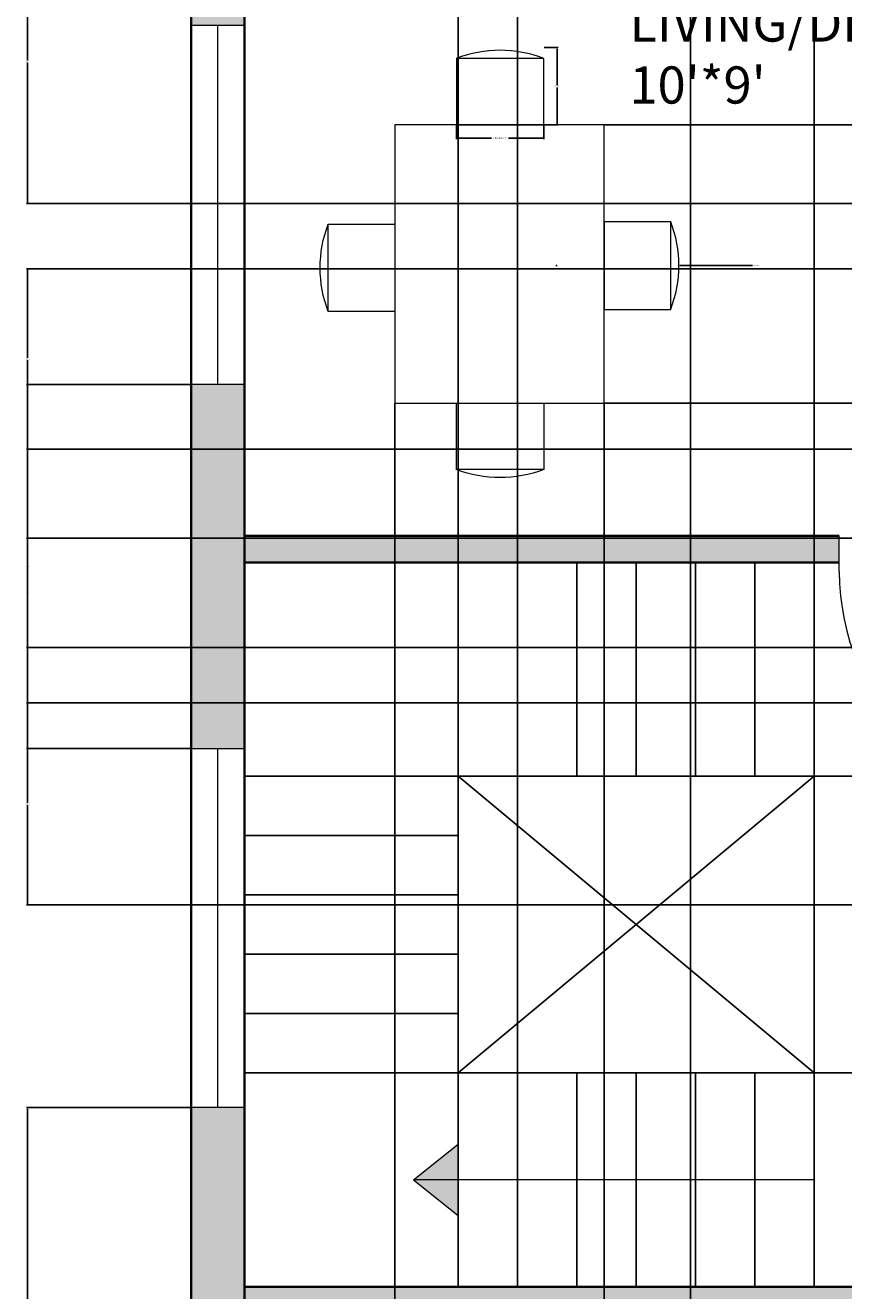
# Model space of a CAD drawing. Units: inches. Extents: x 1841 to 2210, y 2173 to 2736.
# Tile 2 of 4: x 1841 to 1979, y 2316 to 2529. Entities that reach past the tile are written whole.
import ezdxf

# ---------------------------------------------------------------- set-up
doc = ezdxf.new("R2010")
doc.units = ezdxf.units.IN
for name, color, linetype, lineweight in [('A-ANNO-DIMS', 2, 'Continuous', 18), ('A-ANNO-SYMB', 7, 'Continuous', 18), ('A-AREA-IDEN', 10, 'Continuous', 18), ('A-FLOR-STRS', 7, 'Continuous', 25), ('A-FURN', 8, 'Continuous', 18), ('A-WALL', 7, 'Continuous', 35), ('A-WALL-PATT', 252, 'Continuous', 13), ('DOOR', 50, 'Continuous', 18), ('WIN', 193, 'Continuous', 18)]:
    doc.layers.add(name, color=color, linetype=linetype, lineweight=lineweight)
doc.styles.get("Standard").update_dxf_attribs({"font": 'arial.ttf'})
doc.dimstyles.get("Standard").update_dxf_attribs({"dimtxt": 0.18, "dimasz": 0.18, "dimexe": 0.18, "dimexo": 0.0625, "dimgap": 0.09, "dimtad": 0, "dimtih": 1, "dimtoh": 1, "dimdec": 4, "dimzin": 0, "dimdsep": 46, "dimtxsty": 'Standard', "dimcen": 0.09, "dimadec": 0, "dimazin": 0, "dimtfac": 1, "dimtdec": 4, "dimtofl": 0, "dimtmove": 0, "dimatfit": 3, "dimfxl": 1, "dimtolj": 1, "dimtzin": 0, "dimarcsym": 0})

# ---------------------------------------------------------------- blocks, each defined once
blk = doc.blocks.new('*U2')
for p, q in [((0, 0), (0, -6)), ((40, 0), (40, -6))]:
    blk.add_line(p, q)
blk.add_lwpolyline([(0, 0), (0, 40), (1.75, 40), (1.75, 0)], close=True)
blk.add_arc((0, 0), 40, 0, 90)
blk = doc.blocks.new('WIN-60IN-NOM')
blk.add_line((4.5, 0), (4.5, 60.52))
blk.add_lwpolyline([(0, 60.52), (9, 60.52), (9, 0), (0, 0)], close=True)
blk = doc.blocks.new('CHAIR-DINING')
blk.add_lwpolyline([(0, 0), (14.75, 0), (14.75, 11.2), (0, 11.2)], close=True)
blk.add_arc((7.37, -8.08), 20.64, 69.065, 110.935)
blk = doc.blocks.new('*D14')
at = {"layer": 'A-ANNO-DIMS', "color": 0, "lineweight": -2, "transparency": 16777216}
for p, q in [((1913.74, 2512.08), (1913.74, 2509.75)), ((1928.49, 2512.08), (1928.49, 2509.75)), ((1913.92, 2509.93), (1919.69, 2509.93)), ((1928.31, 2509.93), (1922.54, 2509.93))]:
    blk.add_line(p, q, dxfattribs=at)
at = {"layer": 'A-ANNO-DIMS', "color": 0, "transparency": 16777216}
for points in [[(1913.92, 2509.96), (1913.92, 2509.9), (1913.74, 2509.93)], [(1928.31, 2509.96), (1928.31, 2509.9), (1928.49, 2509.93)]]:
    blk.add_solid(points, dxfattribs=at)
at = {"layer": 'Defpoints', "color": 0, "transparency": 16777216}
for p in [(1913.74, 2512.15), (1928.49, 2512.15), (1928.49, 2509.93)]:
    blk.add_point(p, dxfattribs=at)
at = {"layer": 'A-ANNO-DIMS', "color": 0, "transparency": 16777216, "insert": (1921.12, 2509.93), "char_height": 0.18, "attachment_point": 5}
blk.add_mtext('\\A1;DINING CHAIR 15 TYP.', dxfattribs=at)
blk = doc.blocks.new('*D15')
at = {"layer": 'A-ANNO-DIMS', "color": 0, "lineweight": -2, "transparency": 16777216}
for p, q in [((1928.55, 2525.16), (1930.88, 2525.16)), ((1930.7, 2524.98), (1930.7, 2518.84)), ((1930.7, 2512.33), (1930.7, 2518.47)), ((1928.55, 2512.15), (1930.88, 2512.15))]:
    blk.add_line(p, q, dxfattribs=at)
at = {"layer": 'A-ANNO-DIMS', "color": 0, "transparency": 16777216}
for points in [[(1930.67, 2524.98), (1930.73, 2524.98), (1930.7, 2525.16)], [(1930.67, 2512.33), (1930.73, 2512.33), (1930.7, 2512.15)]]:
    blk.add_solid(points, dxfattribs=at)
at = {"layer": 'Defpoints', "color": 0, "transparency": 16777216}
for p in [(1928.49, 2525.16), (1930.7, 2525.16), (1928.49, 2512.15)]:
    blk.add_point(p, dxfattribs=at)
at = {"layer": 'A-ANNO-DIMS', "color": 0, "transparency": 16777216, "insert": (1930.7, 2518.65), "char_height": 0.18, "attachment_point": 5}
blk.add_mtext('\\A1;13 TYP.', dxfattribs=at)
blk = doc.blocks.new('*D29')
at = {"layer": 'A-ANNO-DIMS', "color": 0, "lineweight": -2, "transparency": 16777216}
for p, q in [((1868.99, 2346.57), (1841.32, 2346.57)), ((1841.5, 2346.39), (1841.5, 2287.67)), ((1841.5, 2228.59), (1841.5, 2287.31)), ((1868.99, 2228.41), (1841.32, 2228.41))]:
    blk.add_line(p, q, dxfattribs=at)
at = {"layer": 'A-ANNO-DIMS', "color": 0, "transparency": 16777216}
for points in [[(1841.47, 2346.39), (1841.53, 2346.39), (1841.5, 2346.57)], [(1841.47, 2228.59), (1841.53, 2228.59), (1841.5, 2228.41)]]:
    blk.add_solid(points, dxfattribs=at)
at = {"layer": 'Defpoints', "color": 0, "transparency": 16777216}
for p in [(1841.5, 2346.57), (1869.05, 2346.57), (1869.05, 2228.41)]:
    blk.add_point(p, dxfattribs=at)
at = {"layer": 'A-ANNO-DIMS', "color": 0, "transparency": 16777216, "insert": (1841.5, 2287.49), "char_height": 0.18, "attachment_point": 5}
blk.add_mtext('\\A1;118.17', dxfattribs=at)
blk = doc.blocks.new('*D30')
at = {"layer": 'A-ANNO-DIMS', "color": 0, "lineweight": -2, "transparency": 16777216}
for p, q in [((1868.99, 2468.41), (1841.32, 2468.41)), ((1841.5, 2468.23), (1841.5, 2437.93)), ((1841.5, 2407.27), (1841.5, 2437.56)), ((1868.99, 2407.09), (1841.32, 2407.09))]:
    blk.add_line(p, q, dxfattribs=at)
at = {"layer": 'A-ANNO-DIMS', "color": 0, "transparency": 16777216}
for points in [[(1841.47, 2468.23), (1841.53, 2468.23), (1841.5, 2468.41)], [(1841.47, 2407.27), (1841.53, 2407.27), (1841.5, 2407.09)]]:
    blk.add_solid(points, dxfattribs=at)
at = {"layer": 'Defpoints', "color": 0, "transparency": 16777216}
for p in [(1841.5, 2468.41), (1869.05, 2468.41), (1869.05, 2407.09)]:
    blk.add_point(p, dxfattribs=at)
at = {"layer": 'A-ANNO-DIMS', "color": 0, "transparency": 16777216, "insert": (1841.5, 2437.75), "char_height": 0.18, "attachment_point": 5}
blk.add_mtext('\\A1;61.32', dxfattribs=at)
blk = doc.blocks.new('*D35')
at = {"layer": 'A-ANNO-DIMS', "color": 0, "lineweight": -2, "transparency": 16777216}
for p, q in [((2159.99, 2546.82), (1841.32, 2546.82)), ((1841.5, 2546.64), (1841.5, 2523.04)), ((1841.5, 2499.09), (1841.5, 2522.68)), ((2159.99, 2498.91), (1841.32, 2498.91))]:
    blk.add_line(p, q, dxfattribs=at)
at = {"layer": 'A-ANNO-DIMS', "color": 0, "transparency": 16777216}
for points in [[(1841.47, 2546.64), (1841.53, 2546.64), (1841.5, 2546.82)], [(1841.47, 2499.09), (1841.53, 2499.09), (1841.5, 2498.91)]]:
    blk.add_solid(points, dxfattribs=at)
at = {"layer": 'Defpoints', "color": 0, "transparency": 16777216}
for p in [(1841.5, 2546.82), (2160.05, 2546.82), (2160.05, 2498.91)]:
    blk.add_point(p, dxfattribs=at)
at = {"layer": 'A-ANNO-DIMS', "color": 0, "transparency": 16777216, "insert": (1841.5, 2522.86), "char_height": 0.18, "attachment_point": 5}
blk.add_mtext('\\A1;47.91', dxfattribs=at)
blk = doc.blocks.new('*D37')
at = {"layer": 'A-ANNO-DIMS', "color": 0, "lineweight": -2, "transparency": 16777216}
for p, q in [((1878.05, 2402.47), (1878.05, 2736.14)), ((1878.23, 2735.96), (1895.83, 2735.96)), ((1913.87, 2735.96), (1896.27, 2735.96)), ((1914.05, 2402.47), (1914.05, 2736.14))]:
    blk.add_line(p, q, dxfattribs=at)
at = {"layer": 'A-ANNO-DIMS', "color": 0, "transparency": 16777216}
for points in [[(1878.23, 2735.99), (1878.23, 2735.93), (1878.05, 2735.96)], [(1913.87, 2735.99), (1913.87, 2735.93), (1914.05, 2735.96)]]:
    blk.add_solid(points, dxfattribs=at)
at = {"layer": 'Defpoints', "color": 0, "transparency": 16777216}
for p in [(1914.05, 2735.96), (1878.05, 2402.41), (1914.05, 2402.41)]:
    blk.add_point(p, dxfattribs=at)
at = {"layer": 'A-ANNO-DIMS', "color": 0, "transparency": 16777216, "insert": (1896.05, 2735.96), "char_height": 0.18, "attachment_point": 5}
blk.add_mtext('\\A1;36', dxfattribs=at)
blk = doc.blocks.new('*D38')
at = {"layer": 'A-ANNO-DIMS', "color": 0, "lineweight": -2, "transparency": 16777216}
for p, q in [((1914.05, 2352.47), (1914.05, 2736.14)), ((1914.23, 2735.96), (1943.83, 2735.96)), ((1973.87, 2735.96), (1944.27, 2735.96)), ((1974.05, 2352.47), (1974.05, 2736.14))]:
    blk.add_line(p, q, dxfattribs=at)
at = {"layer": 'A-ANNO-DIMS', "color": 0, "transparency": 16777216}
for points in [[(1914.23, 2735.99), (1914.23, 2735.93), (1914.05, 2735.96)], [(1973.87, 2735.99), (1973.87, 2735.93), (1974.05, 2735.96)]]:
    blk.add_solid(points, dxfattribs=at)
at = {"layer": 'Defpoints', "color": 0, "transparency": 16777216}
for p in [(1974.05, 2735.96), (1914.05, 2352.41), (1974.05, 2352.41)]:
    blk.add_point(p, dxfattribs=at)
at = {"layer": 'A-ANNO-DIMS', "color": 0, "transparency": 16777216, "insert": (1944.05, 2735.96), "char_height": 0.18, "attachment_point": 5}
blk.add_mtext('\\A1;60', dxfattribs=at)
blk = doc.blocks.new('*D39')
at = {"layer": 'A-ANNO-DIMS', "color": 0, "lineweight": -2, "transparency": 16777216}
for p, q in [((1914.11, 2402.41), (2196.78, 2402.41)), ((2196.6, 2402.23), (2196.6, 2377.59)), ((2196.6, 2352.59), (2196.6, 2377.22)), ((1914.11, 2352.41), (2196.78, 2352.41))]:
    blk.add_line(p, q, dxfattribs=at)
at = {"layer": 'A-ANNO-DIMS', "color": 0, "transparency": 16777216}
for points in [[(2196.57, 2402.23), (2196.63, 2402.23), (2196.6, 2402.41)], [(2196.57, 2352.59), (2196.63, 2352.59), (2196.6, 2352.41)]]:
    blk.add_solid(points, dxfattribs=at)
at = {"layer": 'Defpoints', "color": 0, "transparency": 16777216}
for p in [(1914.05, 2402.41), (2196.6, 2402.41), (1914.05, 2352.41)]:
    blk.add_point(p, dxfattribs=at)
at = {"layer": 'A-ANNO-DIMS', "color": 0, "transparency": 16777216, "insert": (2196.6, 2377.41), "char_height": 0.18, "attachment_point": 5}
blk.add_mtext('\\A1;50', dxfattribs=at)
blk = doc.blocks.new('*D40')
at = {"layer": 'A-ANNO-DIMS', "color": 0, "lineweight": -2, "transparency": 16777216}
for p, q in [((1903.36, 2465.22), (1903.36, 2180.68)), ((1938.67, 2465.22), (1938.67, 2180.68)), ((1903.54, 2180.86), (1920.64, 2180.86)), ((1938.49, 2180.86), (1921.39, 2180.86))]:
    blk.add_line(p, q, dxfattribs=at)
at = {"layer": 'A-ANNO-DIMS', "color": 0, "transparency": 16777216}
for points in [[(1903.54, 2180.89), (1903.54, 2180.83), (1903.36, 2180.86)], [(1938.49, 2180.89), (1938.49, 2180.83), (1938.67, 2180.86)]]:
    blk.add_solid(points, dxfattribs=at)
at = {"layer": 'Defpoints', "color": 0, "transparency": 16777216}
for p in [(1903.36, 2465.28), (1938.67, 2465.28), (1938.67, 2180.86)]:
    blk.add_point(p, dxfattribs=at)
at = {"layer": 'A-ANNO-DIMS', "color": 0, "transparency": 16777216, "insert": (1921.01, 2180.86), "char_height": 0.18, "attachment_point": 5}
blk.add_mtext('\\A1;35.31', dxfattribs=at)
blk = doc.blocks.new('*D41')
at = {"layer": 'A-ANNO-DIMS', "color": 0, "lineweight": -2, "transparency": 16777216}
for p, q in [((1938.73, 2512.15), (2196.78, 2512.15)), ((2196.6, 2511.97), (2196.6, 2488.89)), ((2196.6, 2465.46), (2196.6, 2488.53)), ((1938.73, 2465.28), (2196.78, 2465.28))]:
    blk.add_line(p, q, dxfattribs=at)
at = {"layer": 'A-ANNO-DIMS', "color": 0, "transparency": 16777216}
for points in [[(2196.57, 2511.97), (2196.63, 2511.97), (2196.6, 2512.15)], [(2196.57, 2465.46), (2196.63, 2465.46), (2196.6, 2465.28)]]:
    blk.add_solid(points, dxfattribs=at)
at = {"layer": 'Defpoints', "color": 0, "transparency": 16777216}
for p in [(1938.67, 2512.15), (2196.6, 2512.15), (1938.67, 2465.28)]:
    blk.add_point(p, dxfattribs=at)
at = {"layer": 'A-ANNO-DIMS', "color": 0, "transparency": 16777216, "insert": (2196.6, 2488.71), "char_height": 0.18, "attachment_point": 5}
blk.add_mtext('\\A1;46.87', dxfattribs=at)
blk = doc.blocks.new('*D42')
at = {"layer": 'A-ANNO-DIMS', "color": 0, "lineweight": -2, "transparency": 16777216}
for p, q in [((1878.05, 2550.84), (1878.05, 2180.68)), ((1953.17, 2550.84), (1953.17, 2180.68)), ((1878.23, 2180.86), (1915.22, 2180.86)), ((1952.99, 2180.86), (1916, 2180.86))]:
    blk.add_line(p, q, dxfattribs=at)
at = {"layer": 'A-ANNO-DIMS', "color": 0, "transparency": 16777216}
for points in [[(1878.23, 2180.89), (1878.23, 2180.83), (1878.05, 2180.86)], [(1952.99, 2180.89), (1952.99, 2180.83), (1953.17, 2180.86)]]:
    blk.add_solid(points, dxfattribs=at)
at = {"layer": 'Defpoints', "color": 0, "transparency": 16777216}
for p in [(1878.05, 2550.91), (1953.17, 2550.91), (1953.17, 2180.86)]:
    blk.add_point(p, dxfattribs=at)
at = {"layer": 'A-ANNO-DIMS', "color": 0, "transparency": 16777216, "insert": (1915.61, 2180.86), "char_height": 0.18, "attachment_point": 5}
blk.add_mtext('\\A1;75.12', dxfattribs=at)
blk = doc.blocks.new('*D44')
at = {"layer": 'A-ANNO-DIMS', "color": 0, "lineweight": -2, "transparency": 16777216}
for p, q in [((2047.49, 2414.75), (1841.32, 2414.75)), ((1841.5, 2414.57), (1841.5, 2397.92)), ((1841.5, 2380.9), (1841.5, 2397.56)), ((2047.49, 2380.72), (1841.32, 2380.72))]:
    blk.add_line(p, q, dxfattribs=at)
at = {"layer": 'A-ANNO-DIMS', "color": 0, "transparency": 16777216}
for points in [[(1841.47, 2414.57), (1841.53, 2414.57), (1841.5, 2414.75)], [(1841.47, 2380.9), (1841.53, 2380.9), (1841.5, 2380.72)]]:
    blk.add_solid(points, dxfattribs=at)
at = {"layer": 'Defpoints', "color": 0, "transparency": 16777216}
for p in [(1841.5, 2414.75), (2047.55, 2414.75), (2047.55, 2380.72)]:
    blk.add_point(p, dxfattribs=at)
at = {"layer": 'A-ANNO-DIMS', "color": 0, "transparency": 16777216, "insert": (1841.5, 2397.74), "char_height": 0.18, "attachment_point": 5}
blk.add_mtext('\\A1;34.03', dxfattribs=at)
blk = doc.blocks.new('*D46')
at = {"layer": 'A-ANNO-DIMS', "color": 0, "lineweight": -2, "transparency": 16777216}
for p, q in [((1914.05, 2316.47), (1914.05, 2736.14)), ((1914.23, 2735.96), (1918.84, 2735.96)), ((1923.87, 2735.96), (1919.26, 2735.96)), ((1924.05, 2316.47), (1924.05, 2736.14))]:
    blk.add_line(p, q, dxfattribs=at)
at = {"layer": 'A-ANNO-DIMS', "color": 0, "transparency": 16777216}
for points in [[(1914.23, 2735.99), (1914.23, 2735.93), (1914.05, 2735.96)], [(1923.87, 2735.99), (1923.87, 2735.93), (1924.05, 2735.96)]]:
    blk.add_solid(points, dxfattribs=at)
at = {"layer": 'Defpoints', "color": 0, "transparency": 16777216}
for p in [(1924.05, 2735.96), (1914.05, 2316.41), (1924.05, 2316.41)]:
    blk.add_point(p, dxfattribs=at)
at = {"layer": 'A-ANNO-DIMS', "color": 0, "transparency": 16777216, "insert": (1919.05, 2735.96), "char_height": 0.18, "attachment_point": 5}
blk.add_mtext('\\A1;10', dxfattribs=at)
blk = doc.blocks.new('*D48')
at = {"layer": 'A-ANNO-DIMS', "color": 0, "lineweight": -2, "transparency": 16777216}
for p, q in [((2066.48, 2442.49), (1841.32, 2442.49)), ((1841.5, 2442.31), (1841.5, 2433.48)), ((1841.5, 2424.29), (1841.5, 2433.12)), ((2066.48, 2424.11), (1841.32, 2424.11))]:
    blk.add_line(p, q, dxfattribs=at)
at = {"layer": 'A-ANNO-DIMS', "color": 0, "transparency": 16777216}
for points in [[(1841.47, 2442.31), (1841.53, 2442.31), (1841.5, 2442.49)], [(1841.47, 2424.29), (1841.53, 2424.29), (1841.5, 2424.11)]]:
    blk.add_solid(points, dxfattribs=at)
at = {"layer": 'Defpoints', "color": 0, "transparency": 16777216}
for p in [(1841.5, 2442.49), (2066.54, 2442.49), (2066.54, 2424.11)]:
    blk.add_point(p, dxfattribs=at)
at = {"layer": 'A-ANNO-DIMS', "color": 0, "transparency": 16777216, "insert": (1841.5, 2433.3), "char_height": 0.18, "attachment_point": 5}
blk.add_mtext('\\A1;18.377', dxfattribs=at)
blk = doc.blocks.new('*D50')
at = {"layer": 'A-ANNO-DIMS', "color": 0, "lineweight": -2, "transparency": 16777216}
for p, q in [((2110.31, 2487.88), (1841.32, 2487.88)), ((1841.5, 2487.7), (1841.5, 2472.88)), ((1841.5, 2457.7), (1841.5, 2472.52)), ((2110.31, 2457.52), (1841.32, 2457.52))]:
    blk.add_line(p, q, dxfattribs=at)
at = {"layer": 'A-ANNO-DIMS', "color": 0, "transparency": 16777216}
for points in [[(1841.47, 2487.7), (1841.53, 2487.7), (1841.5, 2487.88)], [(1841.47, 2457.7), (1841.53, 2457.7), (1841.5, 2457.52)]]:
    blk.add_solid(points, dxfattribs=at)
at = {"layer": 'Defpoints', "color": 0, "transparency": 16777216}
for p in [(1841.5, 2487.88), (2110.38, 2487.88), (2110.38, 2457.52)]:
    blk.add_point(p, dxfattribs=at)
at = {"layer": 'A-ANNO-DIMS', "color": 0, "transparency": 16777216, "insert": (1841.5, 2472.7), "char_height": 0.18, "attachment_point": 5}
blk.add_mtext('\\A1;30.36', dxfattribs=at)
blk = doc.blocks.new('*D54')
at = {"layer": 'A-ANNO-DIMS', "color": 0, "lineweight": -2, "transparency": 16777216}
for p, q in [((1930.5, 2488.44), (1930.68, 2488.44)), ((1930.59, 2488.35), (1930.59, 2488.53)), ((1963.61, 2488.44), (1951.41, 2488.44))]:
    blk.add_line(p, q, dxfattribs=at)
at = {"layer": 'A-ANNO-DIMS', "color": 0, "transparency": 16777216}
blk.add_solid([(1951.41, 2488.47), (1951.41, 2488.41), (1951.23, 2488.44)], dxfattribs=at)
at = {"layer": 'Defpoints', "color": 0, "transparency": 16777216}
for p in [(1930.59, 2488.44), (1951.23, 2488.44)]:
    blk.add_point(p, dxfattribs=at)
at = {"layer": 'A-ANNO-DIMS', "color": 0, "transparency": 16777216, "insert": (1964.29, 2488.44), "char_height": 0.18, "attachment_point": 5}
blk.add_mtext('\\A1;2X R20.64', dxfattribs=at)

msp = doc.modelspace()

# ---------------------------------------------------------------- hatches: boundary and pattern name
at = {"layer": 'A-ANNO-SYMB'}
h = msp.add_hatch(color=256, dxfattribs=at)
h.dxf.hatch_style = 1
h.paths.add_polyline_path([(1914.0509, 2340.3926), (1906.5264, 2334.4052), (1914.0509, 2334.4052)])
h.paths.add_polyline_path([(1914.0509, 2334.4052), (1906.5264, 2334.4052), (1914.0509, 2328.4179)])
at = {"layer": 'A-WALL-PATT'}
h = msp.add_hatch(color=256, dxfattribs=at)
h.dxf.hatch_style = 1
h.paths.add_polyline_path([(2169.0509, 2546.8192), (2160.3559, 2546.8192), (2160.3559, 2545.451), (2160.3559, 2529.1476), (2160.0509, 2237.4052), (2128.1686, 2237.4052), (2128.1686, 2228.4052), (2169.0509, 2228.4052)])
h.paths.add_polyline_path([(2067.6527, 2237.4052), (2028.5509, 2237.4052), (2028.5509, 2228.4052), (2067.6527, 2228.4052)])
h.paths.add_polyline_path([(2033.0509, 2321.9228), (2028.5509, 2321.9228), (2028.5509, 2237.4052), (2033.0509, 2237.4052)])
h.paths.add_polyline_path([(2160.0509, 2369.9052), (2052.0509, 2369.9052), (2052.0509, 2380.7227), (2047.5509, 2380.7227), (2047.5509, 2369.9052), (2028.5509, 2369.9052), (2028.5509, 2364.1588), (2028.5509, 2361.9228), (2033.0509, 2361.9228), (2033.0509, 2365.4052), (2050.3181, 2365.4052), (2160.0509, 2365.4052)])
h.paths.add_polyline_path([(1878.0509, 2346.5722), (1869.0509, 2346.5722), (1869.0509, 2228.4052), (1878.0509, 2228.4052), (1878.0509, 2237.4052)])
h.paths.add_polyline_path([(1981.8009, 2316.4052), (1878.0509, 2316.4052), (1878.0509, 2311.9052), (1981.8009, 2311.9052)])
h.paths.add_polyline_path([(1978.2584, 2442.9052), (1878.0509, 2442.9052), (1878.0509, 2438.4052), (1914.0509, 2438.4052), (1978.2584, 2438.4052)])
h.paths.add_polyline_path([(1878.0509, 2468.4052), (1869.0509, 2468.4052), (1869.0509, 2407.0881), (1878.0509, 2407.0881), (1878.0509, 2438.4052)])
h.paths.add_polyline_path([(2028.5509, 2442.9052), (2018.2584, 2442.9052), (2018.2584, 2438.4052), (2028.5509, 2438.4052)])
h.paths.add_polyline_path([(2131.5968, 2498.9052), (2002.5509, 2498.9052), (2002.5509, 2500.7487), (1998.0509, 2500.7487), (1998.0509, 2494.4052), (2131.5968, 2494.4052)])
h.paths.add_polyline_path([(2033.0509, 2489.9052), (2033.0509, 2494.4052), (2028.5509, 2494.4052), (2028.5509, 2489.9052), (2028.5509, 2417.9052), (2131.5509, 2417.9052), (2131.5509, 2422.4052), (2033.0509, 2422.4052), (2033.0294, 2446.4052)])
h.paths.add_polyline_path([(1953.1667, 2555.4052), (1878.0509, 2555.4052), (1878.0509, 2550.9052), (1953.1667, 2550.9052)], flags=17)
h.paths.add_polyline_path([(1878.0509, 2699.4052), (2160.0509, 2699.4052), (2160.0509, 2607.3351), (2169.0509, 2607.3351), (2169.0509, 2708.4052), (1869.0509, 2708.4052), (1869.0509, 2528.9211), (1878.0509, 2528.9211), (1878.0509, 2550.9052), (1878.0509, 2555.4052)])
h.paths.add_polyline_path([(1998.0509, 2555.4052), (1993.1667, 2555.4052), (1993.1667, 2550.9052), (1998.0509, 2550.9052)], flags=17)
h.paths.add_polyline_path([(2002.5509, 2550.9052), (1998.0509, 2550.9052), (1998.0509, 2540.7487), (2002.5509, 2540.7487)], flags=17)
h.paths.add_polyline_path([(2002.5509, 2576.8157), (2002.5509, 2607.2805), (2002.5509, 2699.4052), (1998.0509, 2699.4052), (1998.0509, 2555.4052), (1998.0509, 2550.9052), (2002.5509, 2550.9052)], flags=17)
h.paths.add_polyline_path([(2160.0509, 2642.4052), (2089.2965, 2642.4052), (2089.2965, 2637.9052), (2160.0509, 2637.9052)], flags=17)
h.paths.add_polyline_path([(2056.0629, 2642.4052), (2054.0509, 2642.4052), (2054.0509, 2699.4052), (2049.5509, 2699.4052), (2049.5509, 2642.4052), (2002.5509, 2642.4052), (2002.5509, 2637.9052), (2054.0509, 2637.9052), (2056.0629, 2637.9052)], flags=17)
h.paths.add_polyline_path([(1924.594, 2243.1802), (1965.0263, 2243.1802), (1965.0263, 2266.5581), (1924.594, 2266.5581)], flags=9)
h.paths.add_polyline_path([(2082.2056, 2327.2752), (2130.8731, 2327.2752), (2130.8731, 2350.6531), (2082.2056, 2350.6531)], flags=9)
h.paths.add_polyline_path([(2000.1077, 2344.9343), (2000.1077, 2400.666), (1976.7298, 2400.666), (1976.7298, 2344.9343)], flags=9)
h.paths.add_polyline_path([(2161.6353, 2440.9897), (2161.6353, 2476.9732), (2138.2574, 2476.9732), (2138.2574, 2440.9897)], flags=24)
h.paths.add_polyline_path([(2044.2273, 2462.409), (2085.775, 2462.409), (2085.775, 2485.7869), (2044.2273, 2485.7869)], flags=25)
h.paths.add_polyline_path([(1940.3738, 2512.1813), (2005.58, 2512.1813), (2005.58, 2535.5592), (1940.3738, 2535.5592)], flags=9)
h.paths.add_polyline_path([(2088.5551, 2604.7497), (2142.0901, 2604.7497), (2142.0901, 2628.1276), (2088.5551, 2628.1276)], flags=25)
h.paths.add_polyline_path([(2110.3045, 2670.6273), (2145.8692, 2670.6273), (2145.8692, 2694.0052), (2110.3045, 2694.0052)], flags=25)
h.paths.add_polyline_path([(2002.7596, 2670.6273), (2043.2176, 2670.6273), (2043.2176, 2694.0052), (2002.7596, 2694.0052)], flags=24)
h.paths.add_polyline_path([(1907.1501, 2670.6273), (1955.8175, 2670.6273), (1955.8175, 2694.0052), (1907.1501, 2694.0052)], flags=25)

# ---------------------------------------------------------------- linework, layer by layer
at = {"layer": 'A-ANNO-SYMB'}
for p, q in [((1906.5264, 2334.4052), (1914.0509, 2340.3926)), ((1974.0509, 2334.4052), (1906.5264, 2334.4052)), ((1906.5264, 2334.4052), (1914.0509, 2328.4179))]:
    msp.add_line(p, q, dxfattribs=at)
at = {"layer": 'A-FLOR-STRS'}
for p, q in [((1878.0509, 2438.4052), (1878.0509, 2402.4052)), ((1878.0509, 2438.4052), (1914.0509, 2438.4052)), ((1914.0509, 2316.4052), (1914.0509, 2438.4052)), ((1924.0509, 2402.4052), (1924.0509, 2438.4052)), ((1934.0509, 2402.4052), (1934.0509, 2438.4052)), ((1944.0509, 2402.4052), (1944.0509, 2438.4052)), ((1954.0509, 2402.4052), (1954.0509, 2438.4052)), ((1964.0509, 2402.4052), (1964.0509, 2438.4052)), ((1914.0509, 2402.4052), (1878.0509, 2402.4052)), ((1914.0509, 2402.4052), (1964.0509, 2402.4052)), ((1914.0509, 2402.4052), (1914.0509, 2352.4052)), ((1914.0509, 2352.4052), (1974.0509, 2402.4052)), ((1914.0509, 2402.4052), (1974.0509, 2352.4052)), ((1914.0509, 2392.4052), (1878.0509, 2392.4052)), ((1914.0509, 2382.4052), (1878.0509, 2382.4052)), ((1914.0509, 2372.4052), (1878.0509, 2372.4052)), ((1914.0509, 2362.4052), (1878.0509, 2362.4052)), ((1914.0509, 2352.4052), (1878.0509, 2352.4052)), ((1974.0509, 2352.4052), (1914.0509, 2352.4052)), ((1914.0509, 2352.4052), (1914.0509, 2316.4052)), ((1924.0509, 2316.4052), (1924.0509, 2352.4052)), ((1934.0509, 2316.4052), (1934.0509, 2352.4052)), ((1944.0509, 2316.4052), (1944.0509, 2352.4052)), ((1954.0509, 2316.4052), (1954.0509, 2352.4052)), ((1964.0509, 2316.4052), (1964.0509, 2352.4052)), ((1974.0509, 2316.4052), (1974.0509, 2352.4052))]:
    msp.add_line(p, q, dxfattribs=at)
msp.add_lwpolyline([(1974.0509, 2352.4052), (1914.0509, 2352.4052), (1914.0509, 2402.4052), (1974.0509, 2402.4052)], close=True, dxfattribs=at)
at = {"layer": 'A-FURN'}
msp.add_lwpolyline([(1903.3594, 2465.2791), (1938.6659, 2465.2791), (1938.6659, 2512.1455), (1903.3594, 2512.1455)], close=True, dxfattribs=at)
at = {"layer": 'A-WALL'}
for p, q in [((1878.0509, 2550.9052), (1878.0509, 2442.9052)), ((1878.0509, 2442.9052), (1978.2584, 2442.9052)), ((1878.0509, 2438.4052), (1978.2584, 2438.4052)), ((1878.0509, 2438.4052), (1978.2584, 2438.4052)), ((1878.0509, 2438.4052), (1878.0509, 2316.4052)), ((1878.0509, 2316.4052), (1981.8009, 2316.4052))]:
    msp.add_line(p, q, dxfattribs=at)
msp.add_lwpolyline([(1869.0509, 2228.4052), (2169.0509, 2228.4052), (2169.0509, 2708.4052), (1869.0509, 2708.4052)], close=True, dxfattribs=at)
msp.add_lwpolyline([(2028.5509, 2237.4052), (2160.0509, 2237.4052), (2160.0509, 2699.4052), (1878.0509, 2699.4052), (1878.0509, 2237.4052)], dxfattribs=at)

# ---------------------------------------------------------------- block references
at = {"layer": 'A-FURN'}
msp.add_blockref('CHAIR-DINING', (1913.741, 2512.145), dxfattribs=at)
at = {"layer": 'A-FURN', "extrusion": (0, 0, -1), "zscale": -1}
for p, rotation in [((-1903.3599, 2495.4308), 269.9999999999988), ((-1913.741, 2465.2795), 180)]:
    msp.add_blockref('CHAIR-DINING', p, dxfattribs=dict(at, rotation=rotation))
at = {"layer": 'A-FURN', "rotation": 269.9999999999988}
msp.add_blockref('CHAIR-DINING', (1938.6655, 2495.8159), dxfattribs=at)
at = {"layer": 'DOOR', "rotation": 180}
msp.add_blockref('*U2', (2018.2584, 2436.9052), dxfattribs=at)
at = {"layer": 'WIN'}
for p in [(1869.051, 2468.405), (1869.051, 2346.572)]:
    msp.add_blockref('WIN-60IN-NOM', p, dxfattribs=at)

# ---------------------------------------------------------------- texts
at = {"layer": 'A-AREA-IDEN', "insert": (1942.893, 2532.4416), "char_height": 6.26506, "attachment_point": 1}
msp.add_mtext_dynamic_manual_height_columns("LIVING/DINING\\P10'*9'", width=112.651532, gutter_width=31.3253, heights=[0], dxfattribs=at)

# ---------------------------------------------------------------- dimensions: what is measured, and where the dimension line sits
at = {"layer": 'A-ANNO-DIMS'}
for base, p1, p2, override, picture, middle in [((1914.0509, 2735.9552), (1878.0509, 2402.4052), (1914.0509, 2402.4052), {"dimdec": 0, "dimlfac": 1, "dimrnd": 0, "dimzin": 0, "dimdsep": 46, "dimlunit": 2}, '*D37', (1896.0509, 2735.9552)), ((1974.0509, 2735.9552), (1914.0509, 2352.4052), (1974.0509, 2352.4052), {"dimdec": 0, "dimlfac": 1, "dimrnd": 0, "dimzin": 0, "dimdsep": 46, "dimlunit": 2}, '*D38', (1944.0509, 2735.9552)), ((1924.0509, 2735.9552), (1914.0509, 2316.4052), (1924.0509, 2316.4052), {"dimdec": 0, "dimlfac": 1, "dimrnd": 0, "dimzin": 0, "dimdsep": 46, "dimlunit": 2}, '*D46', (1919.0509, 2735.9552)), ((1953.1667, 2180.8552), (1878.0509, 2550.9052), (1953.1667, 2550.9052), {"dimdec": 2, "dimlfac": 1, "dimrnd": 0, "dimzin": 0, "dimdsep": 46, "dimlunit": 2}, '*D42', (1915.6088, 2180.8552)), ((1938.6659, 2180.8552), (1903.3594, 2465.2791), (1938.6659, 2465.2791), {"dimdec": 2, "dimlfac": 1, "dimrnd": 0, "dimzin": 0, "dimdsep": 46, "dimlunit": 2}, '*D40', (1921.0127, 2180.8552))]:
    dim = msp.add_linear_dim(base=base, p1=p1, p2=p2, dimstyle='Standard', override=override, dxfattribs=at)
    dim.commit()
    dim.dimension.update_dxf_attribs({"geometry": picture, "text_midpoint": middle})
for base, p1, p2, override, picture, middle in [((1841.5009, 2546.8192), (2160.0509, 2498.9052), (2160.0509, 2546.8192), {"dimdec": 2, "dimlfac": 1, "dimrnd": 0, "dimzin": 0, "dimdsep": 46, "dimlunit": 2}, '*D35', (1841.5009, 2522.8622)), ((2196.6009, 2512.1455), (1938.6659, 2465.2791), (1938.6659, 2512.1455), {"dimdec": 2, "dimlfac": 1, "dimrnd": 0, "dimzin": 0, "dimdsep": 46, "dimlunit": 2}, '*D41', (2196.6009, 2488.7123)), ((1841.5009, 2487.8791), (2110.3763, 2457.5216), (2110.3763, 2487.8791), {"dimdec": 2, "dimlfac": 1, "dimrnd": 0, "dimzin": 0, "dimdsep": 46, "dimlunit": 2}, '*D50', (1841.5009, 2472.7004)), ((1841.5009, 2468.4052), (1869.0509, 2407.0881), (1869.0509, 2468.4052), {"dimdec": 2, "dimlfac": 1, "dimrnd": 0, "dimzin": 0, "dimdsep": 46, "dimlunit": 2}, '*D30', (1841.5009, 2437.7467)), ((1841.5009, 2442.4893), (2066.5401, 2424.1127), (2066.5401, 2442.4893), {"dimdec": 3, "dimlfac": 1, "dimrnd": 0, "dimzin": 0, "dimdsep": 46, "dimlunit": 2}, '*D48', (1841.5009, 2433.301)), ((1841.5009, 2414.752), (2047.5509, 2380.7227), (2047.5509, 2414.752), {"dimdec": 2, "dimlfac": 1, "dimrnd": 0, "dimzin": 0, "dimdsep": 46, "dimlunit": 2}, '*D44', (1841.5009, 2397.7374)), ((2196.6009, 2402.4052), (1914.0509, 2352.4052), (1914.0509, 2402.4052), {"dimdec": 0, "dimlfac": 1, "dimrnd": 0, "dimzin": 0, "dimdsep": 46, "dimlunit": 2}, '*D39', (2196.6009, 2377.4052)), ((1841.5009, 2346.5722), (1869.0509, 2228.4052), (1869.0509, 2346.5722), {"dimdec": 2, "dimlfac": 1, "dimrnd": 0, "dimzin": 0, "dimdsep": 46, "dimlunit": 2}, '*D29', (1841.5009, 2287.4887))]:
    dim = msp.add_linear_dim(base=base, p1=p1, p2=p2, angle=90, dimstyle='Standard', override=override, dxfattribs=at)
    dim.commit()
    dim.dimension.update_dxf_attribs({"geometry": picture, "text_midpoint": middle})
dim = msp.add_linear_dim(base=(1930.7038, 2525.1623), p1=(1928.4912, 2512.1455), p2=(1928.4912, 2525.1623), angle=90, text='<> TYP.', dimstyle='Standard', override={"dimdec": 0, "dimlfac": 1, "dimrnd": 0, "dimzin": 0, "dimdsep": 46, "dimlunit": 2}, dxfattribs=at)
dim.commit()
dim.dimension.update_dxf_attribs({"geometry": '*D15', "text_midpoint": (1930.7038, 2518.6539)})
dim = msp.add_linear_dim(base=(1928.4912, 2509.9329), p1=(1913.7405, 2512.1455), p2=(1928.4912, 2512.1455), text='DINING CHAIR <> TYP.', dimstyle='Standard', override={"dimdec": 0, "dimlfac": 1, "dimrnd": 0, "dimzin": 0, "dimdsep": 46, "dimlunit": 2}, dxfattribs=at)
dim.commit()
dim.dimension.update_dxf_attribs({"geometry": '*D14', "text_midpoint": (1921.1159, 2509.9329)})
dim = msp.add_radius_dim(center=(1930.5872, 2488.441), mpoint=(1951.2286, 2488.441), text='2X <>', dimstyle='Standard', override={"dimdec": 2, "dimlfac": 1, "dimrnd": 0, "dimzin": 0, "dimdsep": 46, "dimlunit": 2}, dxfattribs=at)
dim.commit()
dim.dimension.update_dxf_attribs({"geometry": '*D54', "text_midpoint": (1963.6134, 2488.441), "dimtype": 164})

doc.saveas('drawing.dxf')
